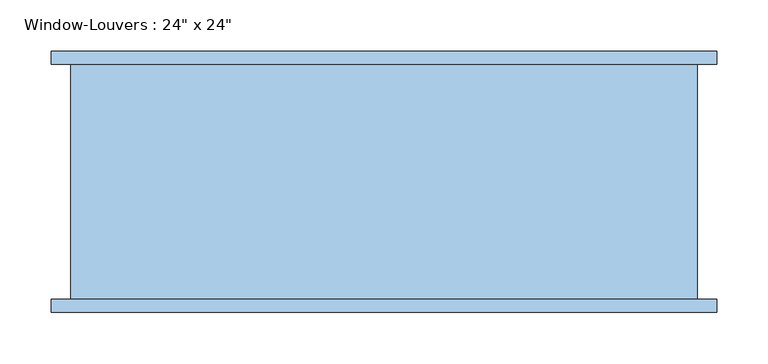
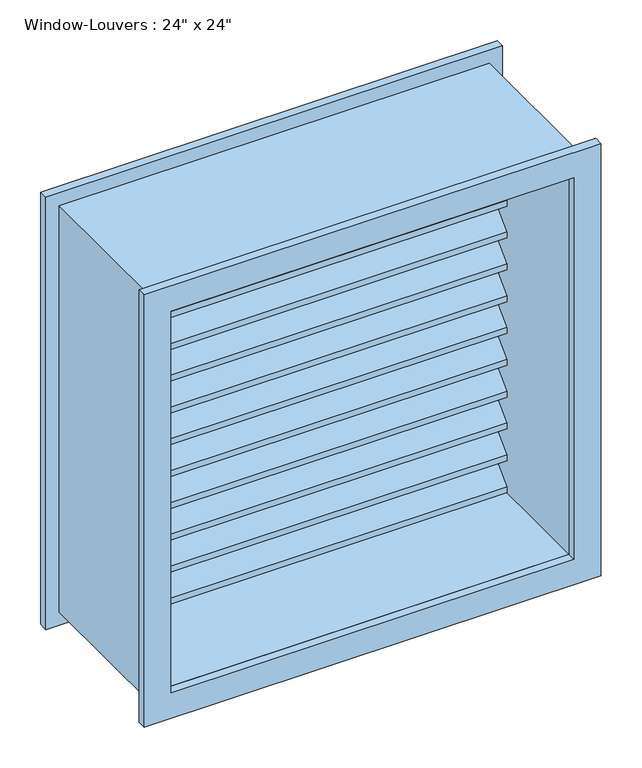
"""IFC4 building model written with IfcOpenShell, lengths in millimetres: window geometry."""

from ifc_helpers import new_model, si_unit, frame, origin, place, context, project, spatial, polyline, outline, extrude, source, transform, mapped, element, save


def window_f2d8fef0(model_context):
    return source(origin(), model_context, "Body", "SweptSolid", [
        extrude(outline(polyline([(107.95, 1419.1754778), (107.95, 1410.1952217), (69.85, 1448.2952217), (31.75, 1410.1952217), (31.75, 1419.1754778), (69.85, 1457.2754778), (107.95, 1419.1754778)])), frame((-285.75, 0.0, 0.0), z_axis=(1.0, 0.0, 0.0), x_axis=(0.0, 1.0, 0.0)), (0.0, 0.0, 1.0), 571.5),
        extrude(outline(polyline([(107.95, 1371.5009557), (107.95, 1362.5206995), (69.85, 1400.6206995), (31.75, 1362.5206995), (31.75, 1371.5009557), (69.85, 1409.6009557), (107.95, 1371.5009557)])), frame((-285.75, 0.0, 0.0), z_axis=(1.0, 0.0, 0.0), x_axis=(0.0, 1.0, 0.0)), (0.0, 0.0, 1.0), 571.5),
        extrude(outline(polyline([(107.95, 1323.8264335), (107.95, 1314.8461774), (69.85, 1352.9461774), (31.75, 1314.8461774), (31.75, 1323.8264335), (69.85, 1361.9264335), (107.95, 1323.8264335)])), frame((-285.75, 0.0, 0.0), z_axis=(1.0, 0.0, 0.0), x_axis=(0.0, 1.0, 0.0)), (0.0, 0.0, 1.0), 571.5),
        extrude(outline(polyline([(107.95, 1276.1519113), (107.95, 1267.1716552), (69.85, 1305.2716552), (31.75, 1267.1716552), (31.75, 1276.1519113), (69.85, 1314.2519113), (107.95, 1276.1519113)])), frame((-285.75, 0.0, 0.0), z_axis=(1.0, 0.0, 0.0), x_axis=(0.0, 1.0, 0.0)), (0.0, 0.0, 1.0), 571.5),
        extrude(outline(polyline([(107.95, 1228.4773891), (107.95, 1219.497133), (69.85, 1257.597133), (31.75, 1219.497133), (31.75, 1228.4773891), (69.85, 1266.5773891), (107.95, 1228.4773891)])), frame((-285.75, 0.0, 0.0), z_axis=(1.0, 0.0, 0.0), x_axis=(0.0, 1.0, 0.0)), (0.0, 0.0, 1.0), 571.5),
        extrude(outline(polyline([(107.95, 1180.802867), (107.95, 1171.8226109), (69.85, 1209.9226109), (31.75, 1171.8226109), (31.75, 1180.802867), (69.85, 1218.902867), (107.95, 1180.802867)])), frame((-285.75, 0.0, 0.0), z_axis=(1.0, 0.0, 0.0), x_axis=(0.0, 1.0, 0.0)), (0.0, 0.0, 1.0), 571.5),
        extrude(outline(polyline([(107.95, 1133.1283448), (107.95, 1124.1480887), (69.85, 1162.2480887), (31.75, 1124.1480887), (31.75, 1133.1283448), (69.85, 1171.2283448), (107.95, 1133.1283448)])), frame((-285.75, 0.0, 0.0), z_axis=(1.0, 0.0, 0.0), x_axis=(0.0, 1.0, 0.0)), (0.0, 0.0, 1.0), 571.5),
        extrude(outline(polyline([(107.95, 1085.4538226), (107.95, 1076.4735665), (69.85, 1114.5735665), (31.75, 1076.4735665), (31.75, 1085.4538226), (69.85, 1123.5538226), (107.95, 1085.4538226)])), frame((-285.75, 0.0, 0.0), z_axis=(1.0, 0.0, 0.0), x_axis=(0.0, 1.0, 0.0)), (0.0, 0.0, 1.0), 571.5),
        extrude(outline(polyline([(107.95, 1037.7793005), (107.95, 1028.7990443), (69.85, 1066.8990443), (31.75, 1028.7990443), (31.75, 1037.7793005), (69.85, 1075.8793005), (107.95, 1037.7793005)])), frame((-285.75, 0.0, 0.0), z_axis=(1.0, 0.0, 0.0), x_axis=(0.0, 1.0, 0.0)), (0.0, 0.0, 1.0), 571.5),
        extrude(outline(polyline([(107.95, 990.1047783), (107.95, 981.1245222), (69.85, 1019.2245222), (31.75, 981.1245222), (31.75, 990.1047783), (69.85, 1028.2047783), (107.95, 990.1047783)])), frame((-285.75, 0.0, 0.0), z_axis=(1.0, 0.0, 0.0), x_axis=(0.0, 1.0, 0.0)), (0.0, 0.0, 1.0), 571.5),
        extrude(outline(polyline([(107.95, 1466.85), (107.95, 1457.8697439), (69.85, 1495.9697439), (31.75, 1457.8697439), (31.75, 1466.85), (69.85, 1504.95), (107.95, 1466.85)])), frame((-285.75, 0.0, 0.0), z_axis=(1.0, 0.0, 0.0), x_axis=(0.0, 1.0, 0.0)), (0.0, 0.0, 1.0), 571.5),
        extrude(outline(polyline([(107.95, 942.4302561), (107.95, 933.45), (69.85, 971.55), (31.75, 933.45), (31.75, 942.4302561), (69.85, 980.5302561), (107.95, 942.4302561)])), frame((-285.75, 0.0, 0.0), z_axis=(1.0, 0.0, 0.0), x_axis=(0.0, 1.0, 0.0)), (0.0, 0.0, 1.0), 571.5),
        extrude(outline(polyline([(1524.0, 304.8), (1524.0, -304.8), (914.4, -304.8), (914.4, 304.8), (1524.0, 304.8)]), holes=[polyline([(1504.95, 285.75), (933.45, 285.75), (933.45, -285.75), (1504.95, -285.75), (1504.95, 285.75)])]), frame((0.0, -120.65, 0.0), z_axis=(0.0, 1.0, 0.0), x_axis=(0.0, 0.0, 1.0)), (0.0, 0.0, 1.0), 228.6),
        extrude(outline(polyline([(1543.05, 323.85), (1543.05, -323.85), (895.35, -323.85), (895.35, 323.85), (1543.05, 323.85)]), holes=[polyline([(1504.95, 285.75), (933.45, 285.75), (933.45, -285.75), (1504.95, -285.75), (1504.95, 285.75)])]), frame((0.0, -133.35, 0.0), z_axis=(0.0, 1.0, 0.0), x_axis=(0.0, 0.0, 1.0)), (0.0, 0.0, 1.0), 12.7),
        extrude(outline(polyline([(1543.05, -323.85), (895.35, -323.85), (895.35, 323.85), (1543.05, 323.85), (1543.05, -323.85)]), holes=[polyline([(1504.95, -285.75), (1504.95, 285.75), (933.45, 285.75), (933.45, -285.75), (1504.95, -285.75)])]), frame((0.0, 107.95, 0.0), z_axis=(0.0, 1.0, 0.0), x_axis=(0.0, 0.0, 1.0)), (0.0, 0.0, 1.0), 12.7),
    ])


if __name__ == "__main__":
    model = new_model("IFC4")
    model_context = context("Model", 3, world=origin())
    ifc_project = project(units=[si_unit("LENGTHUNIT", "METRE", prefix="MILLI")], contexts=[model_context])
    site = spatial("IfcSite", under=ifc_project)
    building = spatial("IfcBuilding", under=site)
    placement = place(None, origin())
    window_shape = window_f2d8fef0(model_context)
    element("IfcWindow", 1, ObjectType="Window-Louvers : 24\" x 24\"", at=placement, inside=building, context=model_context, shape_type="MappedRepresentation", body=[
        mapped(window_shape, transform((0.0, 0.0, 0.0), x_axis=(1.0, 0.0, 0.0), y_axis=(0.0, 1.0, 0.0), z_axis=(0.0, 0.0, 1.0))),
    ])
    save(model, "model.ifc")

# Revit data of these elements
# Type "Window-Louvers : 24\" x 24\""
#   Type Mark = "21"
#   Construction Type Id = "GSP4R"
#   Assembly Code = "B20"
#   Analytic Construction = "1/8 in Pilkington single glazing"
#   Visual Light Transmittance = 0.9
#   Thermal Resistance (R) = 1.53941 (h·ft²·°F)/BTU
#   Solar Heat Gain Coefficient = 0.78
#   Max Height = 1' - 11.74264"
#   Height = 2' - 0"
#   Heat Transfer Coefficient (U) = 0.6496 BTU/(h·ft²·°F)
#   Blade Width [instance default] = 1' - 10 1/2"
#   Blade Vertical Thickness = 0' - 0.35355"
#   Blade Thickness = 0' - 0 1/4"
#   Blade Spacing = 0' - 1 1/2"
#   Blade Height = 0' - 1.85355"
#   Blade Depth = 0' - 3"
#   Blade Angle = 45.00°
#   Default Sill Height = 3' - 0"
#   Trim Projection_Exterior = 0' - 0 1/2"
#   Trim Projection_Interior = 0' - 0 1/2"
#   Trim Width_Exterior = 0' - 1 1/2"
#   Trim Width_Interior = 0' - 1 1/2"
#   Width = 2' - 0"
#   Max Blade Count = 12
#   Define Thermal Properties by = 1
#   Blade Count = 12
#   Frame Material = Birch
#   Louver Material = Birch
#   Trim Exterior Material = Birch
#   Trim Interior Material = Birch
#   Wall Closure = (empty or 0)
# Element 1 (IfcWindow, "Window-Louvers : 24\" x 24\"")
#   Materials on its faces: "Birch"
# Materials
#   "Birch": class "Wood", colour RGB 224 178 126, transparency 0, Description = "Betula Alleghaniensis", Cost = 0
